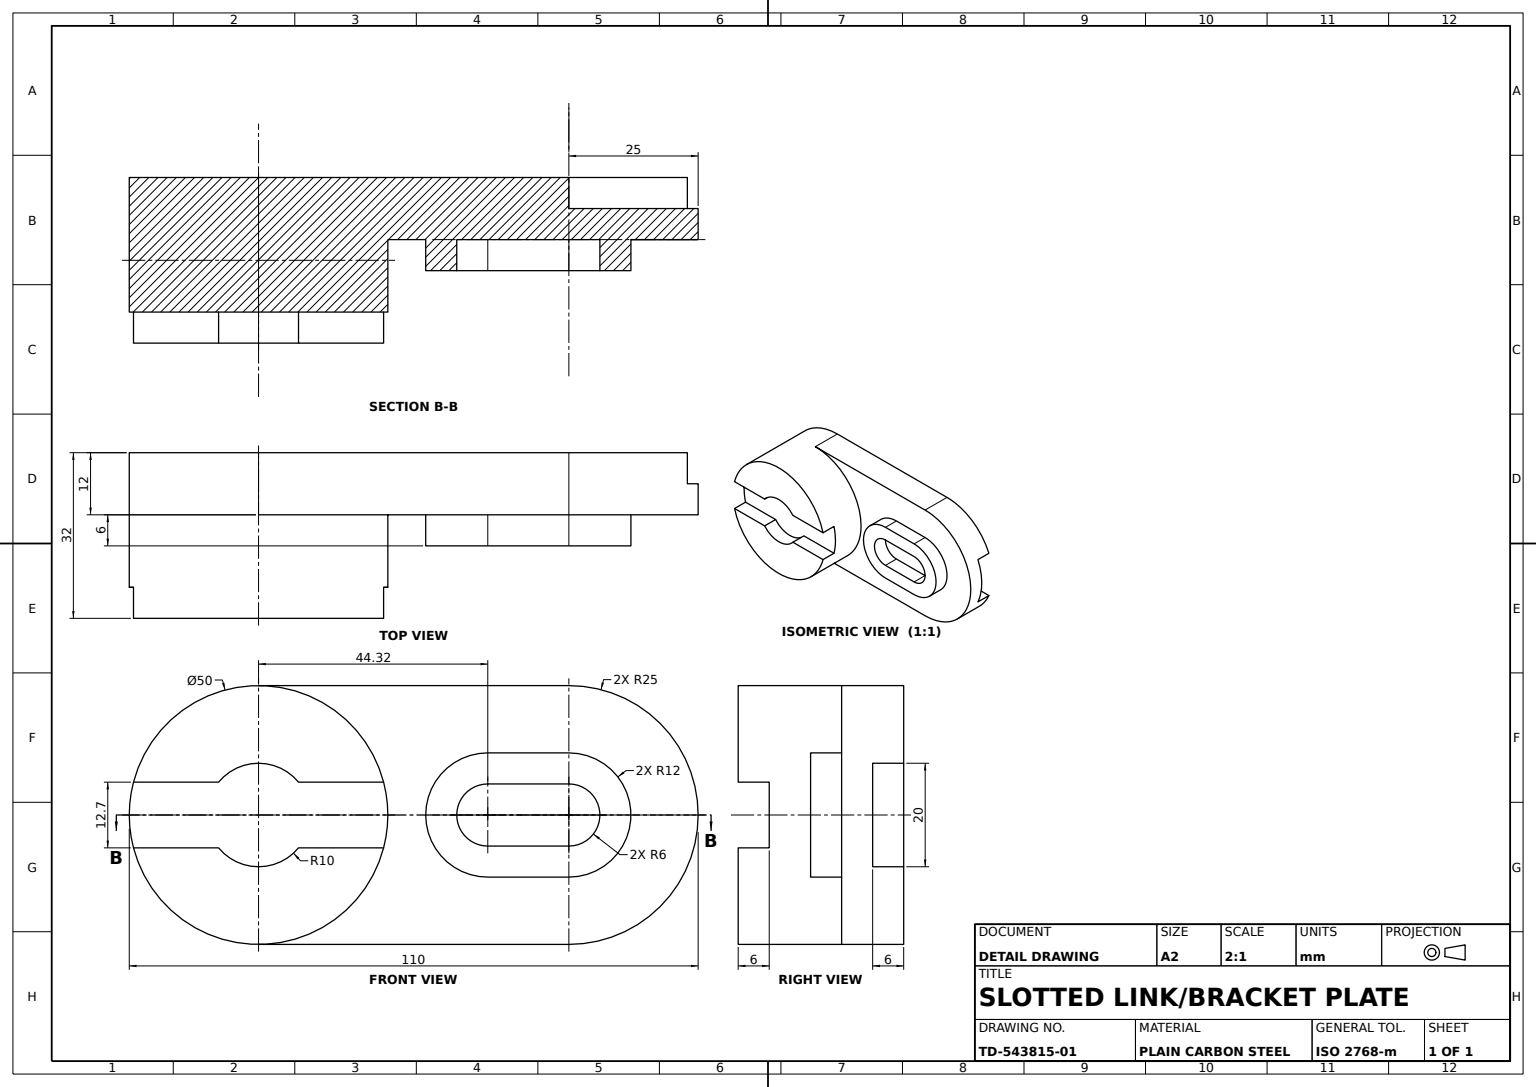
from build123d import *

# Parameters (mm, degrees)
BASE_PLATE_DEPTH          = 12
HUB_BOSS_SKETCH_R         = 25
HUB_BOSS_DEPTH            = 20
HUB_START                 = -6
HUB_KEYHOLE_SLOT_SKETCH_R = 10
HUB_KEYHOLE_SLOT_DEPTH    = 6
SLOT_RIM_DEPTH            = 6
OBROUND_SLOT_DEPTH        = 95.201910809
OBROUND_SLOT_DEPTH_BACK   = 6


with BuildPart() as part:
    # Base Plate Sketch → Base Plate (new body)
    with BuildSketch(Plane.XY):
        with BuildLine():
            Line((0, 25), (60, 25))
            ThreePointArc((60, 25), (85, 0), (60, -25))
            Line((60, -25), (0, -25))
            ThreePointArc((0, -25), (-25, 0), (0, 25))
        make_face()
    extrude(amount=BASE_PLATE_DEPTH)

    # Hub Boss Sketch → Hub Boss (add)
    with BuildSketch(Plane.XY.offset(12)):
        with Locations(Location((0, 0, 0), (0, 0, 270))):
            Circle(HUB_BOSS_SKETCH_R)
    extrude(amount=HUB_BOSS_DEPTH)

    # Hub Keyhole Slot Sketch → Hub Keyhole Slot (cut)
    with BuildSketch(Plane.XY.offset(32).offset(HUB_START)):
        with BuildLine():
            ThreePointArc((-7.726954142, -6.347769662), (-10, 0), (-7.726954142, 6.347769662))
            Line((-7.726954142, 6.347769662), (-24.180691064, 6.347769662))
            ThreePointArc((-24.180691064, 6.347769662), (-25, 0), (-24.180691064, -6.347769662))
            Line((-24.180691064, -6.347769662), (-7.726954142, -6.347769662))
        make_face()
        Circle(HUB_KEYHOLE_SLOT_SKETCH_R)
        with BuildLine():
            Line((24.180691064, 6.347769662), (7.726954142, 6.347769662))
            ThreePointArc((7.726954142, 6.347769662), (9.414604119, 3.371235573), (10, 0))
            ThreePointArc((10, 0), (9.414604119, -3.371235573), (7.726954142, -6.347769662))
            Line((7.726954142, -6.347769662), (24.180691064, -6.347769662))
            ThreePointArc((24.180691064, -6.347769662), (24.794326736, -3.200212759), (25, 0))
            ThreePointArc((25, 0), (24.794326736, 3.200212759), (24.180691064, 6.347769662))
        make_face()
    extrude(amount=HUB_KEYHOLE_SLOT_DEPTH, mode=Mode.SUBTRACT)

    # Slot Rim Sketch → Slot Rim (add)
    with BuildSketch(Plane.XY.offset(12)):
        with BuildLine():
            Line((44.323016702, 12), (60, 12))
            ThreePointArc((60, 12), (72, 0), (60, -12))
            Line((60, -12), (44.323016702, -12))
            ThreePointArc((44.323016702, -12), (32.323016702, 0), (44.323016702, 12))
        make_face()
        with BuildLine():
            Line((44.323016702, 6), (60, 6))
            ThreePointArc((60, 6), (66, 0), (60, -6))
            Line((60, -6), (44.323016702, -6))
            ThreePointArc((44.323016702, -6), (38.323016702, 0), (44.323016702, 6))
        make_face(mode=Mode.SUBTRACT)
    extrude(amount=SLOT_RIM_DEPTH)

    # Obround Slot Sketch → Obround Slot (cut, two sides: drawn at the far end of the back side and taken through both)
    with BuildSketch(Plane(origin=(0, 0, 0), x_dir=(-1, 0, 0), z_dir=(0, 0, -1)).offset(-OBROUND_SLOT_DEPTH_BACK)):
        with BuildLine():
            ThreePointArc((-82.912878475, 10), (-85, 0), (-82.912878475, -10))
            Line((-82.912878475, -10), (-60, -10))
            Line((-60, -10), (-60, 10))
            Line((-60, 10), (-82.912878475, 10))
        make_face()
    extrude(amount=OBROUND_SLOT_DEPTH + OBROUND_SLOT_DEPTH_BACK, mode=Mode.SUBTRACT)


solid = part.part
